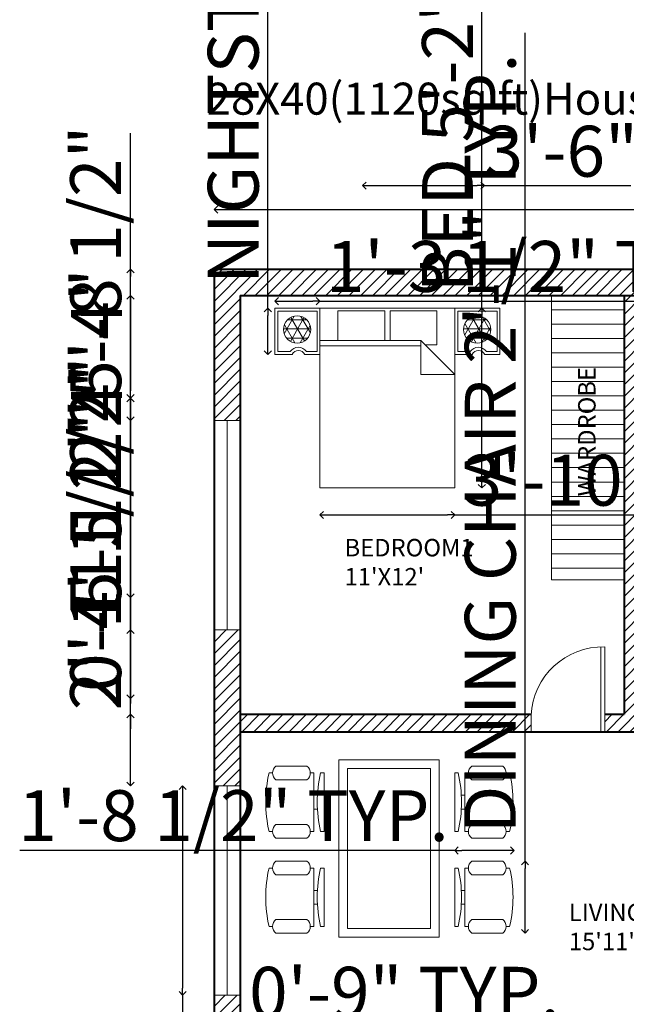
# Model space of a CAD drawing. Units: inches. Extents: x 597 to 1323, y 1833 to 2686.
# Tile 5 of 10: x 705 to 914, y 2171 to 2509. Entities that reach past the tile are written whole.
import ezdxf

# ---------------------------------------------------------------- set-up
doc = ezdxf.new("R2010")
doc.units = ezdxf.units.IN
for name, color, linetype, lineweight in [('A-ANNO-DIMS', 2, 'Continuous', 18), ('A-ANNO-TEXT', 7, 'Continuous', 18), ('A-AREA-IDEN', 7, 'Continuous', 18), ('A-DOOR', 5, 'Continuous', 20), ('A-FLOR-CASE', 8, 'Continuous', 20), ('A-FLOR-CASE-PATT', 8, 'Continuous', 13), ('A-FURN', 8, 'Continuous', 18), ('A-GLAZ', 2, 'Continuous', 18), ('A-WALL', 7, 'Continuous', 40), ('A-WALL-PATT', 8, 'Continuous', 13), ('BEDS', 6, 'Continuous', 18)]:
    doc.layers.add(name, color=color, linetype=linetype, lineweight=lineweight)
doc.styles.get("Standard").update_dxf_attribs({"font": 'arial.ttf'})
doc.dimstyles.new('ISO-25', dxfattribs={"dimtxt": 17.5, "dimasz": 2.5, "dimexe": 0, "dimexo": 0, "dimtad": 1, "dimdec": 1, "dimlunit": 3, "dimtxsty": 'Standard', "dimblk": 'OPEN90', "dimcen": 2.5, "dimadec": 0, "dimazin": 0, "dimtfac": 1, "dimtdec": 1, "dimtmove": 0, "dimatfit": 3, "dimfxl": 0, "dimfxlon": 1, "dimarcsym": 0})

# ---------------------------------------------------------------- blocks, each defined once
blk = doc.blocks.new('Chair - Desk')
for p, q in [((-8.5, 0), (-8.5, -1)), ((-8.5, 0), (8.5, 0)), ((8.5, 0), (8.5, -1)), ((-2, -3), (-2, -1.9355)), ((2, -1.9576), (2, -3)), ((-10.5, -5), (-10.5, -14)), ((-8.5, -3), (-8.5, -4)), ((-8.5, -3), (8.5, -3)), ((-6.5, -14), (-6.5, -5)), ((6.5, -5), (6.5, -14)), ((8.5, -3), (8.5, -4)), ((10.5, -14), (10.5, -5)), ((-8.5, -15), (-8.5, -16)), ((8.5, -15), (8.5, -16))]:
    blk.add_line(p, q)
for centre, radius, start, end in [((0, 34.625), 36.625, 256.5803, 283.4197), ((-8.5, -6.5), 2.5, 36.8699, 143.1301), ((8.5, -6.5), 2.5, 36.8699, 143.1301), ((-8.5, -12.5), 2.5, 216.8699, 323.1301), ((8.5, -12.5), 2.5, 216.8699, 323.1301), ((0, 19.625), 36.625, 256.5803, 283.4197)]:
    blk.add_arc(centre, radius, start, end)
blk = doc.blocks.new('Bed - Queen')
for p, q in [((0, -80.00003), (0, 0)), ((0, 0), (59.99999, 0)), ((59.99999, 0), (59.99999, -80.00003)), ((7.99999, -1.2), (28.79998, -1.2)), ((7.99999, -14.4), (7.99999, -1.2)), ((28.79998, -1.2), (28.79998, -14.4)), ((31.19999, -1.2), (51.99999, -1.2)), ((31.19999, -14.4), (31.19999, -1.2)), ((51.99999, -1.2), (51.99999, -16.4)), ((0, -14.4), (44.8, -14.4)), ((44.8, -16.8), (0, -16.8)), ((59.99999, -29.6), (44.8, -14.4)), ((44.8, -14.4), (44.8, -29.6)), ((51.99999, -16.4), (46.79936, -16.4)), ((44.8, -29.6), (59.99999, -29.6)), ((59.99999, -80.00003), (0, -80.00003))]:
    blk.add_line(p, q)
blk = doc.blocks.new('_Open90')
at = {"color": 0, "linetype": 'ByBlock', "lineweight": -2}
for p, q in [((0, 0), (-1, 0)), ((-0.5, 0.5), (0, 0)), ((0, 0), (-0.5, -0.5))]:
    blk.add_line(p, q, dxfattribs=at)
blk = doc.blocks.new('*D21')
at = {"layer": 'A-ANNO-DIMS', "color": 0, "lineweight": -2, "transparency": 16777216}
blk.add_line((774.39, 2444.15), (1105.39, 2444.15), dxfattribs=at)
at = {"layer": 'Defpoints', "color": 0, "transparency": 16777216}
for p in [(1107.89, 2444.15), (771.89, 2423.61), (1107.89, 2423.61)]:
    blk.add_point(p, dxfattribs=at)
at = {"layer": 'A-ANNO-DIMS', "color": 0, "lineweight": -2, "transparency": 16777216, "xscale": 2.5, "yscale": 2.5, "zscale": 2.5, "rotation": 180}
blk.add_blockref('_Open90', (771.89, 2444.15), dxfattribs=at)
at = {"layer": 'A-ANNO-DIMS', "color": 0, "lineweight": -2, "transparency": 16777216, "xscale": 2.5, "yscale": 2.5, "zscale": 2.5}
blk.add_blockref('_Open90', (1107.89, 2444.15), dxfattribs=at)
at = {"layer": 'A-ANNO-DIMS', "color": 0, "transparency": 16777216, "insert": (939.89, 2453.71), "char_height": 17.5, "attachment_point": 5}
blk.add_mtext("28'", dxfattribs=at)
blk = doc.blocks.new('DOOR-SINGLE-SWING')
for p, q in [((24, 29.15), (24, 0)), ((25.29, 0), (25.29, 29.15)), ((0, 5.64), (0, 0))]:
    blk.add_line(p, q)
blk.add_arc((24.64, 4.49), 24.67, 88.5063, 177.3274)
blk = doc.blocks.new('NIGHTSTAND')
h = blk.add_hatch()
h.set_pattern_fill('NET3', color=256)
h.set_pattern_definition([(0, (-854.688, -2394.344), (0, 3.175), []), (60, (-854.688, -2394.344), (-2.7496307, 1.5875), []), (120, (-854.688, -2394.344), (-2.7496307, -1.5875), [])])
h.paths.add_polyline_path([(12.33, 8.55, 1), (2.97, 8.55, 1)])
for points in [[(5.9, 0), (0, 0), (0, 15.92), (15.5, 15.92), (15.5, 0), (10.29, 0, 0.602187)], [(5.24, 1), (1, 1), (1, 14.92), (14.5, 14.92), (14.5, 1), (10.87, 1, 0.518163)]]:
    blk.add_lwpolyline(points, format="xyb", close=True)
blk.add_circle((7.65, 8.55), 4.68)
blk = doc.blocks.new('WINDOW-72IN')
for p, q in [((0, 0), (0, 9)), ((72, 0), (72, 9)), ((0, 4.5), (72, 4.5))]:
    blk.add_line(p, q)
blk = doc.blocks.new('*D31')
at = {"layer": 'A-ANNO-DIMS', "color": 0, "lineweight": -2, "transparency": 16777216}
for p, q in [((878.8, 2220.09), (878.8, 2504.86)), ((878.8, 2197.8), (878.8, 2217.59))]:
    blk.add_line(p, q, dxfattribs=at)
at = {"layer": 'Defpoints', "color": 0, "transparency": 16777216}
for p in [(875.08, 2220.09), (878.8, 2220.09), (875.08, 2195.3)]:
    blk.add_point(p, dxfattribs=at)
at = {"layer": 'A-ANNO-DIMS', "color": 0, "lineweight": -2, "transparency": 16777216, "xscale": 2.5, "yscale": 2.5, "zscale": 2.5}
for p, rotation in [((878.8, 2220.09), 90), ((878.8, 2195.3), 270)]:
    blk.add_blockref('_Open90', p, dxfattribs=dict(at, rotation=rotation))
at = {"layer": 'A-ANNO-DIMS', "color": 0, "transparency": 16777216, "insert": (869.12, 2363.73), "char_height": 17.5, "attachment_point": 5, "rotation": 90}
blk.add_mtext('DINING CHAIR 2\'-1" TYP.', dxfattribs=at)
blk = doc.blocks.new('*D32')
at = {"layer": 'A-ANNO-DIMS', "color": 0, "lineweight": -2, "transparency": 16777216}
for p, q in [((854.62, 2223.81), (705.07, 2223.81)), ((872.58, 2223.81), (857.12, 2223.81))]:
    blk.add_line(p, q, dxfattribs=at)
at = {"layer": 'Defpoints', "color": 0, "transparency": 16777216}
for p in [(854.62, 2223.81), (854.62, 2220.09), (875.08, 2220.09)]:
    blk.add_point(p, dxfattribs=at)
at = {"layer": 'A-ANNO-DIMS', "color": 0, "lineweight": -2, "transparency": 16777216, "xscale": 2.5, "yscale": 2.5, "zscale": 2.5, "rotation": 180}
blk.add_blockref('_Open90', (854.62, 2223.81), dxfattribs=at)
at = {"layer": 'A-ANNO-DIMS', "color": 0, "lineweight": -2, "transparency": 16777216, "xscale": 2.5, "yscale": 2.5, "zscale": 2.5}
blk.add_blockref('_Open90', (875.08, 2223.81), dxfattribs=at)
at = {"layer": 'A-ANNO-DIMS', "color": 0, "transparency": 16777216, "insert": (778.59, 2233.48), "char_height": 17.5, "attachment_point": 5}
blk.add_mtext('1\'-8 1/2" TYP.', dxfattribs=at)
blk = doc.blocks.new('*D33')
at = {"layer": 'A-ANNO-DIMS', "color": 0, "lineweight": -2, "transparency": 16777216}
for p, q in [((790.41, 2410.26), (790.41, 2685.53)), ((790.41, 2396.84), (790.41, 2407.76))]:
    blk.add_line(p, q, dxfattribs=at)
at = {"layer": 'Defpoints', "color": 0, "transparency": 16777216}
for p in [(790.41, 2410.26), (792.8, 2410.26), (792.8, 2394.34)]:
    blk.add_point(p, dxfattribs=at)
at = {"layer": 'A-ANNO-DIMS', "color": 0, "lineweight": -2, "transparency": 16777216, "xscale": 2.5, "yscale": 2.5, "zscale": 2.5}
for p, rotation in [((790.41, 2410.26), 90), ((790.41, 2394.34), 270)]:
    blk.add_blockref('_Open90', p, dxfattribs=dict(at, rotation=rotation))
at = {"layer": 'A-ANNO-DIMS', "color": 0, "transparency": 16777216, "insert": (780.74, 2549.15), "char_height": 17.5, "attachment_point": 5, "rotation": 90}
blk.add_mtext('NIGHTSTAND 1\'-4" TYP.', dxfattribs=at)
blk = doc.blocks.new('*D34')
at = {"layer": 'A-ANNO-DIMS', "color": 0, "lineweight": -2, "transparency": 16777216}
for p, q in [((795.3, 2412.65), (805.8, 2412.65)), ((808.3, 2412.65), (957.85, 2412.65))]:
    blk.add_line(p, q, dxfattribs=at)
at = {"layer": 'Defpoints', "color": 0, "transparency": 16777216}
for p in [(808.3, 2412.65), (792.8, 2410.26), (808.3, 2410.26)]:
    blk.add_point(p, dxfattribs=at)
at = {"layer": 'A-ANNO-DIMS', "color": 0, "lineweight": -2, "transparency": 16777216, "xscale": 2.5, "yscale": 2.5, "zscale": 2.5, "rotation": 180}
blk.add_blockref('_Open90', (792.8, 2412.65), dxfattribs=at)
at = {"layer": 'A-ANNO-DIMS', "color": 0, "lineweight": -2, "transparency": 16777216, "xscale": 2.5, "yscale": 2.5, "zscale": 2.5}
blk.add_blockref('_Open90', (808.3, 2412.65), dxfattribs=at)
at = {"layer": 'A-ANNO-DIMS', "color": 0, "transparency": 16777216, "insert": (884.33, 2422.33), "char_height": 17.5, "attachment_point": 5}
blk.add_mtext('1\'-3 1/2" TYP.', dxfattribs=at)
blk = doc.blocks.new('*D35')
at = {"layer": 'A-ANNO-DIMS', "color": 0, "lineweight": -2, "transparency": 16777216}
for p, q in [((761.09, 2243.49), (761.09, 2176.49)), ((761.09, 2173.99), (761.09, 1948.8))]:
    blk.add_line(p, q, dxfattribs=at)
at = {"layer": 'Defpoints', "color": 0, "transparency": 16777216}
for p in [(771.89, 2245.99), (761.09, 2173.99), (771.89, 2173.99)]:
    blk.add_point(p, dxfattribs=at)
at = {"layer": 'A-ANNO-DIMS', "color": 0, "lineweight": -2, "transparency": 16777216, "xscale": 2.5, "yscale": 2.5, "zscale": 2.5}
for p, rotation in [((761.09, 2245.99), 90), ((761.09, 2173.99), 270)]:
    blk.add_blockref('_Open90', p, dxfattribs=dict(at, rotation=rotation))
at = {"layer": 'A-ANNO-DIMS', "color": 0, "transparency": 16777216, "insert": (751.41, 2060.14), "char_height": 17.5, "attachment_point": 5, "rotation": 90}
blk.add_mtext('WINDOW 6\'-0" TYP.', dxfattribs=at)
blk = doc.blocks.new('*D36')
at = {"layer": 'A-ANNO-DIMS', "color": 0, "lineweight": -2, "transparency": 16777216}
for p, q in [((774.39, 2163.19), (778.39, 2163.19)), ((780.89, 2163.19), (891.31, 2163.19))]:
    blk.add_line(p, q, dxfattribs=at)
at = {"layer": 'Defpoints', "color": 0, "transparency": 16777216}
for p in [(771.89, 2173.99), (780.89, 2173.99), (780.89, 2163.19)]:
    blk.add_point(p, dxfattribs=at)
at = {"layer": 'A-ANNO-DIMS', "color": 0, "lineweight": -2, "transparency": 16777216, "xscale": 2.5, "yscale": 2.5, "zscale": 2.5, "rotation": 180}
blk.add_blockref('_Open90', (771.89, 2163.19), dxfattribs=at)
at = {"layer": 'A-ANNO-DIMS', "color": 0, "lineweight": -2, "transparency": 16777216, "xscale": 2.5, "yscale": 2.5, "zscale": 2.5}
blk.add_blockref('_Open90', (780.89, 2163.19), dxfattribs=at)
at = {"layer": 'A-ANNO-DIMS', "color": 0, "transparency": 16777216, "insert": (837.35, 2172.75), "char_height": 17.5, "attachment_point": 5}
blk.add_mtext('0\'-9" TYP.', dxfattribs=at)
blk = doc.blocks.new('*D41')
at = {"layer": 'A-ANNO-DIMS', "color": 0, "lineweight": -2, "transparency": 16777216}
for p, q in [((863.97, 2410.26), (863.97, 2576.96)), ((863.97, 2350.91), (863.97, 2407.76))]:
    blk.add_line(p, q, dxfattribs=at)
at = {"layer": 'Defpoints', "color": 0, "transparency": 16777216}
for p in [(854.69, 2410.26), (863.97, 2410.26), (854.69, 2348.41)]:
    blk.add_point(p, dxfattribs=at)
at = {"layer": 'A-ANNO-DIMS', "color": 0, "lineweight": -2, "transparency": 16777216, "xscale": 2.5, "yscale": 2.5, "zscale": 2.5}
for p, rotation in [((863.97, 2410.26), 90), ((863.97, 2348.41), 270)]:
    blk.add_blockref('_Open90', p, dxfattribs=dict(at, rotation=rotation))
at = {"layer": 'A-ANNO-DIMS', "color": 0, "transparency": 16777216, "insert": (854.41, 2494.86), "char_height": 17.5, "attachment_point": 5, "rotation": 90}
blk.add_mtext('BED 5\'-2" TYP.', dxfattribs=at)
blk = doc.blocks.new('*D42')
at = {"layer": 'A-ANNO-DIMS', "color": 0, "lineweight": -2, "transparency": 16777216}
for p, q in [((810.8, 2339.13), (852.19, 2339.13)), ((854.69, 2339.13), (1019.47, 2339.13))]:
    blk.add_line(p, q, dxfattribs=at)
at = {"layer": 'Defpoints', "color": 0, "transparency": 16777216}
for p in [(808.3, 2348.41), (854.69, 2348.41), (854.69, 2339.13)]:
    blk.add_point(p, dxfattribs=at)
at = {"layer": 'A-ANNO-DIMS', "color": 0, "lineweight": -2, "transparency": 16777216, "xscale": 2.5, "yscale": 2.5, "zscale": 2.5, "rotation": 180}
blk.add_blockref('_Open90', (808.3, 2339.13), dxfattribs=at)
at = {"layer": 'A-ANNO-DIMS', "color": 0, "lineweight": -2, "transparency": 16777216, "xscale": 2.5, "yscale": 2.5, "zscale": 2.5}
blk.add_blockref('_Open90', (854.69, 2339.13), dxfattribs=at)
at = {"layer": 'A-ANNO-DIMS', "color": 0, "transparency": 16777216, "insert": (938.33, 2348.81), "char_height": 17.5, "attachment_point": 5}
blk.add_mtext('3\'-10 1/2" TYP.', dxfattribs=at)
blk = doc.blocks.new('*D55')
at = {"layer": 'A-ANNO-DIMS', "color": 0, "lineweight": -2, "transparency": 16777216}
for p, q in [((825.39, 2452.36), (862.39, 2452.36)), ((864.89, 2452.36), (915.14, 2452.36))]:
    blk.add_line(p, q, dxfattribs=at)
at = {"layer": 'Defpoints', "color": 0, "transparency": 16777216}
for p in [(864.89, 2452.36), (822.89, 2075.33), (864.89, 2075.33)]:
    blk.add_point(p, dxfattribs=at)
at = {"layer": 'A-ANNO-DIMS', "color": 0, "lineweight": -2, "transparency": 16777216, "xscale": 2.5, "yscale": 2.5, "zscale": 2.5, "rotation": 180}
blk.add_blockref('_Open90', (822.89, 2452.36), dxfattribs=at)
at = {"layer": 'A-ANNO-DIMS', "color": 0, "lineweight": -2, "transparency": 16777216, "xscale": 2.5, "yscale": 2.5, "zscale": 2.5}
blk.add_blockref('_Open90', (864.89, 2452.36), dxfattribs=at)
at = {"layer": 'A-ANNO-DIMS', "color": 0, "transparency": 16777216, "insert": (891.27, 2461.93), "char_height": 17.5, "attachment_point": 5}
blk.add_mtext('3\'-6"', dxfattribs=at)
blk = doc.blocks.new('*D59')
at = {"layer": 'A-ANNO-DIMS', "color": 0, "lineweight": -2, "transparency": 16777216}
for p, q in [((910.39, 1912.53), (907.89, 1912.53)), ((912.89, 1912.53), (918.89, 1912.53)), ((921.39, 1912.53), (971.66, 1912.53))]:
    blk.add_line(p, q, dxfattribs=at)
at = {"layer": 'Defpoints', "color": 0, "transparency": 16777216}
for p in [(912.89, 2270.61), (918.89, 2264.61), (918.89, 1912.53)]:
    blk.add_point(p, dxfattribs=at)
at = {"layer": 'A-ANNO-DIMS', "color": 0, "lineweight": -2, "transparency": 16777216, "xscale": 2.5, "yscale": 2.5, "zscale": 2.5}
blk.add_blockref('_Open90', (912.89, 1912.53), dxfattribs=at)
at = {"layer": 'A-ANNO-DIMS', "color": 0, "lineweight": -2, "transparency": 16777216, "xscale": 2.5, "yscale": 2.5, "zscale": 2.5, "rotation": 180}
blk.add_blockref('_Open90', (918.89, 1912.53), dxfattribs=at)
at = {"layer": 'A-ANNO-DIMS', "color": 0, "transparency": 16777216, "insert": (947.77, 1922.09), "char_height": 17.5, "attachment_point": 5}
blk.add_mtext('0\'-6"', dxfattribs=at)
blk = doc.blocks.new('*D60')
at = {"layer": 'A-ANNO-DIMS', "color": 0, "lineweight": -2, "transparency": 16777216}
blk.add_line((743.14, 2374.11), (743.14, 2421.11), dxfattribs=at)
at = {"layer": 'Defpoints', "color": 0, "transparency": 16777216}
for p in [(743.14, 2423.61), (771.89, 2423.61), (771.89, 2371.61)]:
    blk.add_point(p, dxfattribs=at)
at = {"layer": 'A-ANNO-DIMS', "color": 0, "lineweight": -2, "transparency": 16777216, "xscale": 2.5, "yscale": 2.5, "zscale": 2.5}
for p, rotation in [((743.14, 2423.61), 90), ((743.14, 2371.61), 270)]:
    blk.add_blockref('_Open90', p, dxfattribs=dict(at, rotation=rotation))
at = {"layer": 'A-ANNO-DIMS', "color": 0, "transparency": 16777216, "insert": (733.76, 2397.61), "char_height": 17.5, "attachment_point": 5, "rotation": 90}
blk.add_mtext('4\'-4"', dxfattribs=at)
blk = doc.blocks.new('*D61')
at = {"layer": 'A-ANNO-DIMS', "color": 0, "lineweight": -2, "transparency": 16777216}
for p, q in [((743.14, 2299.61), (743.14, 2391.36)), ((743.14, 2248.49), (743.14, 2297.11))]:
    blk.add_line(p, q, dxfattribs=at)
at = {"layer": 'Defpoints', "color": 0, "transparency": 16777216}
for p in [(743.14, 2299.61), (771.89, 2299.61), (771.89, 2245.99)]:
    blk.add_point(p, dxfattribs=at)
at = {"layer": 'A-ANNO-DIMS', "color": 0, "lineweight": -2, "transparency": 16777216, "xscale": 2.5, "yscale": 2.5, "zscale": 2.5}
for p, rotation in [((743.14, 2299.61), 90), ((743.14, 2245.99), 270)]:
    blk.add_blockref('_Open90', p, dxfattribs=dict(at, rotation=rotation))
at = {"layer": 'A-ANNO-DIMS', "color": 0, "transparency": 16777216, "insert": (733.46, 2346.74), "char_height": 17.5, "attachment_point": 5, "rotation": 90}
blk.add_mtext('4\'-5 1/2"', dxfattribs=at)
blk = doc.blocks.new('*D69')
at = {"layer": 'A-ANNO-DIMS', "color": 0, "lineweight": -2, "transparency": 16777216}
for p, q in [((743.14, 2412.11), (743.14, 2381.8)), ((743.14, 2379.3), (743.14, 2274.36))]:
    blk.add_line(p, q, dxfattribs=at)
at = {"layer": 'Defpoints', "color": 0, "transparency": 16777216}
for p in [(978.89, 2414.61), (743.14, 2379.3), (978.89, 2379.3)]:
    blk.add_point(p, dxfattribs=at)
at = {"layer": 'A-ANNO-DIMS', "color": 0, "lineweight": -2, "transparency": 16777216, "xscale": 2.5, "yscale": 2.5, "zscale": 2.5}
for p, rotation in [((743.14, 2414.61), 90), ((743.14, 2379.3), 270)]:
    blk.add_blockref('_Open90', p, dxfattribs=dict(at, rotation=rotation))
at = {"layer": 'A-ANNO-DIMS', "color": 0, "transparency": 16777216, "insert": (733.46, 2325.58), "char_height": 17.5, "attachment_point": 5, "rotation": 90}
blk.add_mtext('2\'-11 1/2"', dxfattribs=at)
blk = doc.blocks.new('*D71')
at = {"layer": 'A-ANNO-DIMS', "color": 0, "lineweight": -2, "transparency": 16777216}
for p, q in [((743.14, 2379.3), (743.14, 2470.35)), ((743.14, 2313.23), (743.14, 2376.8))]:
    blk.add_line(p, q, dxfattribs=at)
at = {"layer": 'Defpoints', "color": 0, "transparency": 16777216}
for p in [(743.14, 2379.3), (1066.43, 2379.3), (1066.43, 2310.73)]:
    blk.add_point(p, dxfattribs=at)
at = {"layer": 'A-ANNO-DIMS', "color": 0, "lineweight": -2, "transparency": 16777216, "xscale": 2.5, "yscale": 2.5, "zscale": 2.5}
for p, rotation in [((743.14, 2379.3), 90), ((743.14, 2310.73), 270)]:
    blk.add_blockref('_Open90', p, dxfattribs=dict(at, rotation=rotation))
at = {"layer": 'A-ANNO-DIMS', "color": 0, "transparency": 16777216, "insert": (733.46, 2426.07), "char_height": 17.5, "attachment_point": 5, "rotation": 90}
blk.add_mtext('5\'-8 1/2"', dxfattribs=at)
blk = doc.blocks.new('*D79')
at = {"layer": 'A-ANNO-DIMS', "color": 0, "lineweight": -2, "transparency": 16777216}
for p, q in [((908.7, 1912.53), (910.39, 1912.53)), ((912.89, 1912.53), (1003.93, 1912.53))]:
    blk.add_line(p, q, dxfattribs=at)
at = {"layer": 'Defpoints', "color": 0, "transparency": 16777216}
for p in [(906.2, 2270.61), (912.89, 2270.61), (912.89, 1912.53)]:
    blk.add_point(p, dxfattribs=at)
at = {"layer": 'A-ANNO-DIMS', "color": 0, "lineweight": -2, "transparency": 16777216, "xscale": 2.5, "yscale": 2.5, "zscale": 2.5, "rotation": 180}
blk.add_blockref('_Open90', (906.2, 1912.53), dxfattribs=at)
at = {"layer": 'A-ANNO-DIMS', "color": 0, "lineweight": -2, "transparency": 16777216, "xscale": 2.5, "yscale": 2.5, "zscale": 2.5}
blk.add_blockref('_Open90', (912.89, 1912.53), dxfattribs=at)
at = {"layer": 'A-ANNO-DIMS', "color": 0, "transparency": 16777216, "insert": (959.66, 1922.21), "char_height": 17.5, "attachment_point": 5}
blk.add_mtext('0\'-6 1/2"', dxfattribs=at)
blk = doc.blocks.new('*D80')
at = {"layer": 'A-ANNO-DIMS', "color": 0, "lineweight": -2, "transparency": 16777216}
for p, q in [((743.14, 2278.5), (743.14, 2369.55)), ((743.14, 2270.61), (743.14, 2276)), ((743.14, 2268.11), (743.14, 2265.61))]:
    blk.add_line(p, q, dxfattribs=at)
at = {"layer": 'Defpoints', "color": 0, "transparency": 16777216}
for p in [(743.14, 2276), (978.89, 2276), (978.89, 2270.61)]:
    blk.add_point(p, dxfattribs=at)
at = {"layer": 'A-ANNO-DIMS', "color": 0, "lineweight": -2, "transparency": 16777216, "xscale": 2.5, "yscale": 2.5, "zscale": 2.5}
for p, rotation in [((743.14, 2276), 270), ((743.14, 2270.61), 90)]:
    blk.add_blockref('_Open90', p, dxfattribs=dict(at, rotation=rotation))
at = {"layer": 'A-ANNO-DIMS', "color": 0, "transparency": 16777216, "insert": (733.46, 2325.27), "char_height": 17.5, "attachment_point": 5, "rotation": 90}
blk.add_mtext('0\'-5 1/2"', dxfattribs=at)

msp = doc.modelspace()

# ---------------------------------------------------------------- hatches: boundary and pattern name
at = {"layer": 'A-FLOR-CASE-PATT'}
h = msp.add_hatch(dxfattribs=at)
h.set_pattern_fill('ANSI31', color=256, scale=1.555256, angle=-45, style=0)
h.paths.add_polyline_path([(887.96, 2316.87), (912.89, 2316.87), (912.89, 2414.61), (887.96, 2414.61)])
at = {"layer": 'A-WALL-PATT'}
h = msp.add_hatch(dxfattribs=at)
h.set_pattern_fill('ANSI31', color=256, scale=0.9)
h.paths.add_polyline_path([(927.93, 2423.61), (771.89, 2423.61), (771.89, 2371.61), (780.89, 2371.61), (780.89, 2414.61), (918.89, 2414.61), (927.93, 2414.61)])
h.paths.add_polyline_path([(1107.89, 2423.61), (1074.89, 2423.61), (1074.89, 2414.61), (1098.89, 2414.61), (1098.89, 2382.26), (1107.89, 2382.26)])
h.paths.add_polyline_path([(1002.89, 2423.61), (963.93, 2423.61), (963.93, 2414.61), (978.89, 2414.61), (1002.89, 2414.61)])
h.paths.add_polyline_path([(918.89, 2414.61), (912.89, 2414.61), (912.89, 2270.61), (906.2, 2270.61), (906.2, 2264.61), (918.89, 2264.61), (918.89, 2318.61), (928.09, 2318.61), (928.09, 2324.61), (918.89, 2324.61)])
h.paths.add_polyline_path([(780.89, 2299.61), (771.89, 2299.61), (771.89, 2245.99), (780.89, 2245.99)])
h.paths.add_polyline_path([(780.89, 2173.99), (771.89, 2173.99), (771.89, 1943.61), (790.26, 1943.61), (790.26, 1952.61), (780.89, 1952.61)])
h.paths.add_polyline_path([(873.89, 1991.61), (887.56, 1991.61), (887.56, 2000.61), (864.89, 2000.61), (864.89, 1952.61), (857.81, 1952.61), (857.81, 1943.61), (873.89, 1943.61)])
h.paths.add_polyline_path([(979.81, 2000.61), (908.62, 2000.61), (908.62, 1991.61), (979.81, 1991.61)])
h.paths.add_polyline_path([(931.89, 2138.61), (938.68, 2138.61), (938.68, 2144.61), (925.89, 2144.61), (925.89, 2000.61), (931.89, 2000.61)])
h.paths.add_polyline_path([(870.89, 2084.61), (874.89, 2084.61), (874.89, 2090.61), (870.89, 2090.61), (870.89, 2144.61), (815.52, 2144.61), (815.52, 2138.61), (864.89, 2138.61), (864.89, 2000.61), (870.89, 2000.61)])
h.paths.add_polyline_path([(925.89, 2090.61), (900.18, 2090.61), (900.18, 2084.61), (925.89, 2084.61)])
h.paths.add_polyline_path([(1107.89, 2051.2), (1098.89, 2051.2), (1098.89, 2000.61), (1047.65, 2000.61), (1047.65, 1991.61), (1107.89, 1991.61)])
h.paths.add_polyline_path([(1107.89, 2181.44), (1098.89, 2181.44), (1098.89, 2109.76), (1107.89, 2109.76)])
h.paths.add_polyline_path([(1098.89, 2144.61), (978.89, 2144.61), (978.89, 2157.94), (972.89, 2157.94), (972.89, 2144.61), (963.97, 2144.61), (963.97, 2138.61), (1098.89, 2138.61)])
h.paths.add_polyline_path([(1107.89, 2310.26), (1098.89, 2310.26), (1098.89, 2227.53), (1107.89, 2227.53)])
h.paths.add_polyline_path([(1098.89, 2270.61), (978.89, 2270.61), (978.89, 2276), (972.89, 2276), (972.89, 2183.23), (978.89, 2183.23), (978.89, 2264.61), (1098.89, 2264.61)])
h.paths.add_polyline_path([(880.91, 2270.61), (780.89, 2270.61), (780.89, 2264.61), (880.91, 2264.61)])
h.paths.add_polyline_path([(978.89, 2414.61), (972.89, 2414.61), (972.89, 2324.61), (961.07, 2324.61), (961.07, 2318.61), (972.89, 2318.61), (972.89, 2301.29), (978.89, 2301.29)])
h.paths.add_polyline_path([(790.26, 2144.61), (780.89, 2144.61), (780.89, 2138.61), (790.26, 2138.61)], flags=17)

# ---------------------------------------------------------------- linework, layer by layer
at = {"layer": 'A-FLOR-CASE'}
for p, q in [((887.96, 2316.87), (887.96, 2414.61)), ((912.89, 2414.61), (887.96, 2414.61)), ((912.89, 2316.87), (887.96, 2316.87))]:
    msp.add_line(p, q, dxfattribs=at)
at = {"layer": 'A-FURN'}
for points in [[(814.78, 2254.96), (849.32, 2254.96), (849.32, 2193.92), (814.78, 2193.92)], [(817.78, 2251.96), (846.32, 2251.96), (846.32, 2196.92), (817.78, 2196.92)]]:
    msp.add_lwpolyline(points, close=True, dxfattribs=at)
at = {"layer": 'A-GLAZ'}
msp.add_line((780.89, 2245.99), (780.89, 2245.99), dxfattribs=at)
at = {"layer": 'A-WALL'}
for p, q in [((771.89, 2423.61), (771.89, 1943.61)), ((771.89, 2423.61), (1107.89, 2423.61)), ((780.89, 2414.61), (780.89, 1952.61)), ((780.89, 2414.61), (918.89, 2414.61)), ((912.89, 2414.61), (912.89, 2270.61)), ((780.89, 2270.61), (880.93, 2270.61)), ((906.2, 2270.61), (912.89, 2270.61)), ((780.89, 2264.61), (918.89, 2264.61))]:
    msp.add_line(p, q, dxfattribs=at)

# ---------------------------------------------------------------- block references
at = {"layer": 'A-DOOR'}
msp.add_blockref('DOOR-SINGLE-SWING', (880.91, 2264.61), dxfattribs=at)
at = {"layer": 'A-FURN', "xscale": 1.180397522766371, "yscale": 1.180397522766371, "zscale": 1.180397522766371}
for p, rotation in [((809.71, 2240.38), 270), ((854.62, 2240.38), 89.99999999999999), ((809.71, 2207.7), 270), ((854.62, 2207.7), 89.99999999999999)]:
    msp.add_blockref('Chair - Desk', p, dxfattribs=dict(at, rotation=rotation))
at = {"layer": 'A-GLAZ'}
for p, rotation in [((771.89, 2371.61), 269.9999999999992), ((771.89, 2245.99), 269.9999999999993)]:
    msp.add_blockref('WINDOW-72IN', p, dxfattribs=dict(at, rotation=rotation))
at = {"layer": 'BEDS'}
for p in [(792.8, 2394.34), (854.69, 2394.34)]:
    msp.add_blockref('NIGHTSTAND', p, dxfattribs=at)
at = {"layer": 'BEDS', "xscale": 0.7731367655098573, "yscale": 0.7731367655098573, "zscale": 0.7731367655098573}
msp.add_blockref('Bed - Queen', (808.3, 2410.26), dxfattribs=at)

# ---------------------------------------------------------------- texts
at = {"layer": 'A-ANNO-TEXT', "insert": (769.38, 2487.77), "char_height": 11, "attachment_point": 1}
msp.add_mtext_dynamic_manual_height_columns('28X40(1120sq ft)House Plan-West face -FP1316', width=624.2346, gutter_width=12.5, heights=[0], dxfattribs=at)
at = {"layer": 'A-AREA-IDEN', "insert": (897.06, 2345.54), "char_height": 6, "attachment_point": 1, "rotation": 90}
msp.add_mtext_dynamic_manual_height_columns('WARDROBE', width=54.7527, gutter_width=12.5, heights=[0], dxfattribs=at)
at = {"layer": 'A-AREA-IDEN', "char_height": 6, "attachment_point": 1}
for s, insert in [("BEDROOM1\\P11'X12'", (816.75, 2330.89)), ('LIVING HLL\\P15\'11"X10\'', (893.87, 2205.49))]:
    msp.add_mtext_dynamic_manual_height_columns(s, width=54.7527, gutter_width=12.5, heights=[0], dxfattribs=dict(at, insert=insert))

# ---------------------------------------------------------------- dimensions: what is measured, and where the dimension line sits
at = {"layer": 'A-ANNO-DIMS'}
for base, p1, p2, angle, text, picture, middle in [((790.41, 2410.26), (792.8, 2394.34), (792.8, 2410.26), 90, 'NIGHTSTAND <> TYP.', '*D33', (780.74, 2549.15)), ((863.966, 2410.2595), (854.6884, 2348.4086), (854.6884, 2410.2595), 90, 'BED <> TYP.', '*D41', (854.406, 2494.8622)), ((878.8, 2220.09), (875.08, 2195.3), (875.08, 2220.09), 90, 'DINING CHAIR <> TYP.', '*D31', (869.12, 2363.73)), ((854.62, 2223.81), (875.08, 2220.09), (854.62, 2220.09), 180, '<> TYP.', '*D32', (778.59, 2233.48)), ((761.09, 2173.99), (771.89, 2245.99), (771.89, 2173.99), 270, 'WINDOW <> TYP.', '*D35', (751.41, 2060.14))]:
    dim = msp.add_linear_dim(base=base, p1=p1, p2=p2, angle=angle, text=text, dimstyle='ISO-25', override={"dimdec": 1, "dimlfac": 1, "dimrnd": 0, "dimzin": 1, "dimdsep": 46, "dimlunit": 4, "dimfrac": 2}, dxfattribs=at)
    dim.commit()
    dim.dimension.update_dxf_attribs({"geometry": picture, "text_midpoint": middle})
for base, p1, p2, override, picture, middle in [((864.89, 2452.36), (822.89, 2075.33), (864.89, 2075.33), {"dimdec": 1, "dimlfac": 1, "dimrnd": 0, "dimzin": 1, "dimdsep": 46, "dimlunit": 4, "dimfrac": 2}, '*D55', (891.27, 2461.93)), ((1107.89, 2444.15), (771.89, 2423.61), (1107.89, 2423.61), {"dimclrd": 0, "dimclre": 0, "dimclrt": 0}, '*D21', (939.89, 2453.71)), ((912.89, 1912.53), (906.2, 2270.61), (912.89, 2270.61), {"dimdec": 1, "dimlfac": 1, "dimrnd": 0, "dimzin": 1, "dimdsep": 46, "dimlunit": 4, "dimfrac": 2}, '*D79', (959.66, 1922.21)), ((918.89, 1912.53), (912.89, 2270.61), (918.89, 2264.61), {"dimdec": 1, "dimlfac": 1, "dimrnd": 0, "dimzin": 1, "dimdsep": 46, "dimlunit": 4, "dimfrac": 2}, '*D59', (947.77, 1922.09))]:
    dim = msp.add_linear_dim(base=base, p1=p1, p2=p2, dimstyle='ISO-25', override=override, dxfattribs=at)
    dim.commit()
    dim.dimension.update_dxf_attribs({"geometry": picture, "text_midpoint": middle})
for base, p1, p2, picture, middle in [((743.14, 2379.3), (1066.43, 2310.73), (1066.43, 2379.3), '*D71', (733.46, 2426.07)), ((743.14, 2423.61), (771.89, 2371.61), (771.89, 2423.61), '*D60', (733.76, 2397.61)), ((743.14, 2379.3), (978.89, 2414.61), (978.89, 2379.3), '*D69', (733.46, 2325.58)), ((743.14, 2299.61), (771.89, 2245.99), (771.89, 2299.61), '*D61', (733.46, 2346.74)), ((743.14, 2276), (978.89, 2270.61), (978.89, 2276), '*D80', (733.46, 2325.27))]:
    dim = msp.add_linear_dim(base=base, p1=p1, p2=p2, angle=90, dimstyle='ISO-25', override={"dimdec": 1, "dimlfac": 1, "dimrnd": 0, "dimzin": 1, "dimdsep": 46, "dimlunit": 4, "dimfrac": 2}, dxfattribs=at)
    dim.commit()
    dim.dimension.update_dxf_attribs({"geometry": picture, "text_midpoint": middle})
for base, p1, p2, picture, middle in [((808.3, 2412.65), (792.8, 2410.26), (808.3, 2410.26), '*D34', (884.33, 2422.33)), ((854.69, 2339.13), (808.3, 2348.41), (854.69, 2348.41), '*D42', (938.33, 2348.81)), ((780.89, 2163.19), (771.89, 2173.99), (780.89, 2173.99), '*D36', (837.35, 2172.75))]:
    dim = msp.add_linear_dim(base=base, p1=p1, p2=p2, text='<> TYP.', dimstyle='ISO-25', override={"dimdec": 1, "dimlfac": 1, "dimrnd": 0, "dimzin": 1, "dimdsep": 46, "dimlunit": 4, "dimfrac": 2}, dxfattribs=at)
    dim.commit()
    dim.dimension.update_dxf_attribs({"geometry": picture, "text_midpoint": middle})

doc.saveas('drawing.dxf')
